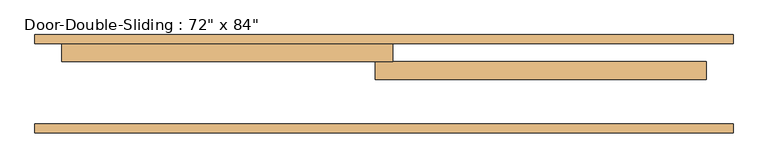
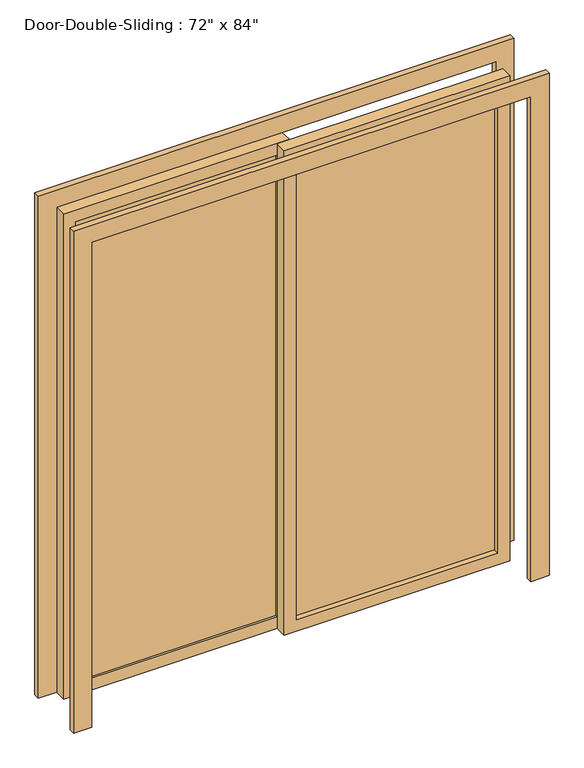
"""IFC4 building model written with IfcOpenShell, lengths in millimetres: door geometry."""

from ifc_helpers import new_model, si_unit, frame, origin, place, context, project, spatial, polyline, outline, extrude, source, transform, mapped, element, save


def door_d4d75d1e(model_context):
    return source(origin(), model_context, "Body", "SweptSolid", [
        extrude(outline(polyline([(0.0, 990.6), (2209.8, 990.6), (2209.8, -990.6), (0.0, -990.6), (0.0, -914.4), (2133.6, -914.4), (2133.6, 914.4), (0.0, 914.4), (0.0, 990.6)])), frame((0.0, 241.3, 0.0), z_axis=(0.0, 1.0, 0.0), x_axis=(0.0, 0.0, 1.0)), (0.0, 0.0, 1.0), 25.4),
        extrude(outline(polyline([(0.0, -990.6), (0.0, -914.4), (2133.6, -914.4), (2133.6, 914.4), (0.0, 914.4), (0.0, 990.6), (2209.8, 990.6), (2209.8, -990.6), (0.0, -990.6)])), frame((0.0, -12.7, 0.0), z_axis=(0.0, 1.0, 0.0), x_axis=(0.0, 0.0, 1.0)), (0.0, 0.0, 1.0), 25.4),
        extrude(outline(polyline([(2133.6, 25.4), (2133.6, -914.4), (0.0, -914.4), (0.0, 25.4), (2133.6, 25.4)]), holes=[polyline([(2082.8, -25.4), (50.8, -25.4), (50.8, -863.6), (2082.8, -863.6), (2082.8, -25.4)])]), frame((0.0, 190.5, 0.0), z_axis=(0.0, 1.0, 0.0), x_axis=(0.0, 0.0, 1.0)), (0.0, 0.0, 1.0), 50.8),
        extrude(outline(polyline([(2133.6, -25.4), (0.0, -25.4), (0.0, 914.4), (2133.6, 914.4), (2133.6, -25.4)]), holes=[polyline([(2082.8, 25.4), (2082.8, 863.6), (50.8, 863.6), (50.8, 25.4), (2082.8, 25.4)])]), frame((0.0, 139.7, 0.0), z_axis=(0.0, 1.0, 0.0), x_axis=(0.0, 0.0, 1.0)), (0.0, 0.0, 1.0), 50.8),
        extrude(outline(polyline([(-25.4, 200.025), (-863.6, 200.025), (-863.6, 206.375), (-25.4, 206.375), (-25.4, 200.025)])), frame((0.0, 0.0, 50.8), z_axis=(0.0, 0.0, 1.0), x_axis=(1.0, 0.0, 0.0)), (0.0, 0.0, 1.0), 2032.0),
        extrude(outline(polyline([(25.4, 168.275), (863.6, 168.275), (863.6, 161.925), (25.4, 161.925), (25.4, 168.275)])), frame((0.0, 0.0, 50.8), z_axis=(0.0, 0.0, 1.0), x_axis=(1.0, 0.0, 0.0)), (0.0, 0.0, 1.0), 2032.0),
    ])


if __name__ == "__main__":
    model = new_model("IFC4")
    model_context = context("Model", 3, world=origin())
    ifc_project = project(units=[si_unit("LENGTHUNIT", "METRE", prefix="MILLI")], contexts=[model_context])
    site = spatial("IfcSite", under=ifc_project)
    building = spatial("IfcBuilding", under=site)
    placement = place(None, origin())
    door_shape = door_d4d75d1e(model_context)
    element("IfcDoor", 1, ObjectType="Door-Double-Sliding : 72\" x 84\"", at=placement, inside=building, context=model_context, shape_type="MappedRepresentation", body=[
        mapped(door_shape, transform((0.0, 0.0, 0.0), x_axis=(1.0, 0.0, 0.0), y_axis=(0.0, 1.0, 0.0), z_axis=(0.0, 0.0, 1.0))),
    ])
    save(model, "model.ifc")

# Revit data of these elements
# Type "Door-Double-Sliding : 72\" x 84\""
#   Type Mark = "12"
#   Construction Type Id = "opn-d45"
#   Assembly Code = "C1020"
#   Analytic Construction = "Wood frame, double glass door "
#   Thickness = 0' - 2"
#   Thermal Resistance (R) = 1.8150 (h·ft²·°F)/BTU
#   Heat Transfer Coefficient (U) = 0.5510 BTU/(h·ft²·°F)
#   Height = 7' - 0"
#   Rail Width = 0' - 2"
#   Stiles = 0' - 2"
#   Trim Projection Ext = 0' - 1"
#   Trim Projection Int = 0' - 1"
#   Trim Width = 0' - 3"
#   Width = 6' - 0"
#   Define Thermal Properties by = 1
#   Glazing = Glass
#   Panel Material = Wood - Birch - Solid Stained Light Low Gloss
#   Trim Material = Paint - Sienna
#   Visual Light Transmittance = 0
#   Solar Heat Gain Coefficient = 0
#   Function = (empty or 0)
#   Wall Closure = (empty or 0)
# Element 1 (IfcDoor, "Door-Double-Sliding : 72\" x 84\"")
#   Materials on its faces: "Paint - Sienna", "Wood - Birch - Solid Stained Light Low Gloss", "Glass"
# Materials
#   "Glass": class "Glass", colour RGB 0 128 192, transparency 0.75, Description = "Soda Lime Glass", Cost = 0
#   "Wood - Birch - Solid Stained Light Low Gloss": class "Wood", colour RGB 210 159 95, transparency 0, Cost = 0
#   "Paint - Sienna": colour RGB 118 70 51, transparency 0, Cost = 0
